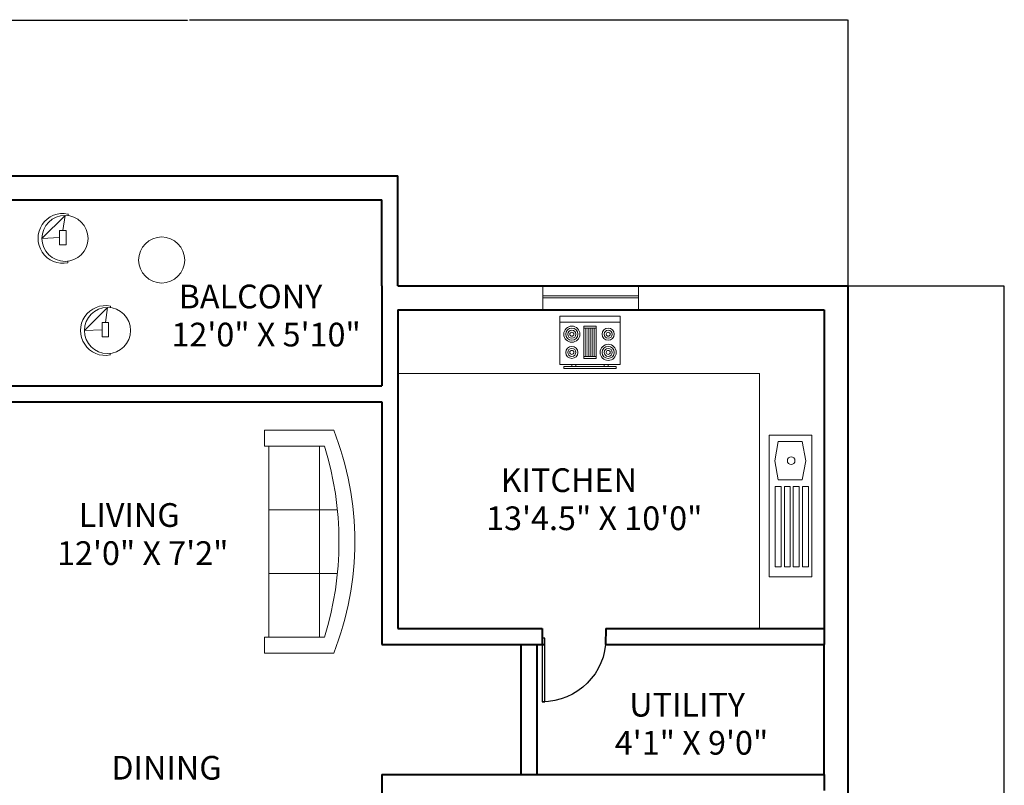
# Model space of a CAD drawing. Units: inches. Extents: x -46 to 1145, y -527 to 760.
# Tile 57 of 57: x 775 to 1145, y 472 to 760. Entities that reach past the tile are written whole.
import ezdxf

# ---------------------------------------------------------------- set-up
doc = ezdxf.new("R2010")
doc.units = ezdxf.units.IN
doc.header["$MEASUREMENT"] = 0
for name, color, linetype, lineweight in [('A-ANNO-DIMS', 2, 'Continuous', 18), ('A-AREA-IDEN', 1, 'Continuous', 18), ('A-EQPM', 2, 'Continuous', 18), ('A-FLOR-CASE', 32, 'Continuous', 18), ('A-FLOR-FIXT', 9, 'Continuous', 18), ('A-FURN', 2, 'Continuous', 13), ('DOORS', 3, 'Continuous', 25), ('WALLS', 4, 'Continuous', 40), ('WINDOWS', 240, 'Continuous', 20)]:
    doc.layers.add(name, color=color, linetype=linetype, lineweight=lineweight)
doc.styles.get("Standard").update_dxf_attribs({"font": 'arial.ttf'})
doc.dimstyles.get("Standard").update_dxf_attribs({"dimtxt": 0.18, "dimasz": 0.18, "dimexe": 0.18, "dimexo": 0.0625, "dimgap": 0.09, "dimtad": 0, "dimtih": 1, "dimtoh": 1, "dimdec": 0, "dimzin": 0, "dimdsep": 46, "dimlunit": 3, "dimtxsty": 'Standard', "dimcen": 0.09, "dimadec": 0, "dimazin": 0, "dimtfac": 1, "dimtdec": 0, "dimtofl": 0, "dimtmove": 0, "dimatfit": 3, "dimfxl": 1, "dimtolj": 1, "dimtzin": 0, "dimarcsym": 0})

# ---------------------------------------------------------------- blocks, each defined once
blk = doc.blocks.new('*U2')
for p, q in [((0, 0), (0, -6)), ((40, 0), (40, -6))]:
    blk.add_line(p, q)
blk.add_lwpolyline([(0, 0), (0, 40), (1.75, 40), (1.75, 0)], close=True)
blk.add_arc((0, 0), 40, 0, 90)
blk = doc.blocks.new('Range-Oven - 30 in top')
for p, q in [((0, -3), (30, -3)), ((12, -6), (18, -6)), ((13, -20), (13, -6)), ((14, -6), (14, -20)), ((15, -20), (15, -6)), ((16, -6), (16, -20)), ((17, -20), (17, -6)), ((6, -24), (6, -25)), ((8, -25), (8, -24)), ((18, -20), (12, -20)), ((22, -25), (22, -24)), ((24, -24), (24, -25))]:
    blk.add_line(p, q)
for points in [[(0, -24), (0, 0), (30, 0), (30, -24)], [(12, -21), (12, -5), (18, -5), (18, -21)], [(2, -26), (2, -25), (28, -25), (28, -26)]]:
    blk.add_lwpolyline(points, close=True)
for centre, radius in [((6, -9), 4), ((6, -9), 3), ((6, -9), 2), ((6, -9), 1), ((24, -9), 3), ((24, -9), 2), ((24, -9), 1), ((24, -18), 4), ((6, -18), 3), ((6, -18), 2), ((6, -18), 1), ((24, -18), 3), ((24, -18), 2), ((24, -18), 1)]:
    blk.add_circle(centre, radius)
blk = doc.blocks.new('Sofa - Roundback 7 ft.')
for p, q in [((-12.00002, -32.4421), (-12.00003, -6.5971)), ((11.99997, -32.4421), (11.99998, -6.5971)), ((-36.000027, -34), (-36.000027, -11.4696)), ((-35.999844, -13.3819), (35.9998, -13.3819)), ((35.99998, -34), (35.99998, -11.4696)), ((-36.000027, -32.4421), (35.99998, -32.4421))]:
    blk.add_line(p, q)
for points in [[(-36.000027, -34), (-42.000027, -34), (-42.000027, -8)], [(41.99998, -8), (41.99998, -34), (35.99998, -34)]]:
    blk.add_lwpolyline(points)
for centre, radius, start, end in [((0, -114.25), 114.25, 68.43141, 111.5686), ((-0.00001, -127.1968), 121.1968, 72.72033, 107.2797)]:
    blk.add_arc(centre, radius, start, end)
blk = doc.blocks.new('SINK-DRAINBOARD')
for p, q in [((3.38, 50.9), (2.09, 43.74)), ((12.47, 50.9), (13.77, 43.74)), ((3.38, 36.58), (2.09, 43.74)), ((12.47, 36.58), (13.77, 43.74))]:
    blk.add_line(p, q)
for points in [[(16.07, 0), (0, 0), (0, 53.35), (16.07, 53.35)], [(4.51, 3.73), (2.3, 3.73), (2.3, 34.08), (4.51, 34.08)], [(7.92, 3.73), (5.72, 3.73), (5.72, 34.08), (7.92, 34.08)], [(11.26, 3.73), (9.05, 3.73), (9.05, 34.08), (11.26, 34.08)], [(14.8, 3.73), (12.59, 3.73), (12.59, 34.08), (14.8, 34.08)]]:
    blk.add_lwpolyline(points, close=True)
for points in [[(3.38, 50.9), (12.47, 50.9)], [(12.47, 36.58), (3.38, 36.58)]]:
    blk.add_lwpolyline(points)
blk.add_circle((8.28, 43.74), 1.44)
blk = doc.blocks.new('BALCONY-CHAIR')
for p, q in [((11.28, 17.97), (11.28, 18.57)), ((1.49, 9.38), (10.16, 18.05)), ((9.33, 12.41), (10.16, 18.05)), ((8.08, 9.69), (1.49, 9.38)), ((11.2, 0.17), (11.2, 0.77))]:
    blk.add_line(p, q)
blk.add_lwpolyline([(10.57, 6.97), (8.08, 6.97), (8.08, 12.41), (10.57, 12.41)], close=True)
blk.add_circle((10.16, 9.38), 8.67)
blk.add_arc((9.38, 9.38), 9.38, 78.3491, 281.1485)
blk = doc.blocks.new('WINDOW-36IN')
for p, q in [((0, 4.5), (0, 9)), ((0, 9), (0, 0)), ((36, 9), (36, 0)), ((0, 5.23), (36, 5.23)), ((0, 4.5), (36, 4.5))]:
    blk.add_line(p, q)
blk = doc.blocks.new('KITCHEN-COUNTER-L')
for p, q in [((136.17, 96), (0, 96)), ((136.17, 24), (136.17, 96)), ((136.17, 0), (136.17, 24))]:
    blk.add_line(p, q)
blk = doc.blocks.new('*D686')
at = {"layer": 'A-ANNO-DIMS', "color": 0, "lineweight": -2, "transparency": 16777216}
for p, q in [((590.06, 659.58), (590.06, 759.67)), ((1086.56, 659.58), (1086.56, 759.67)), ((590.24, 759.49), (837.92, 759.49)), ((1086.38, 759.49), (838.71, 759.49))]:
    blk.add_line(p, q, dxfattribs=at)
at = {"layer": 'A-ANNO-DIMS', "color": 0, "transparency": 16777216}
for points in [[(590.24, 759.52), (590.24, 759.46), (590.06, 759.49)], [(1086.38, 759.52), (1086.38, 759.46), (1086.56, 759.49)]]:
    blk.add_solid(points, dxfattribs=at)
at = {"layer": 'Defpoints', "color": 0, "transparency": 16777216}
for p in [(1086.56, 759.49), (590.06, 659.52), (1086.56, 659.52)]:
    blk.add_point(p, dxfattribs=at)
at = {"layer": 'A-ANNO-DIMS', "color": 0, "transparency": 16777216, "insert": (838.31, 759.49), "char_height": 0.18, "attachment_point": 5}
blk.add_mtext('\\A1;496.5', dxfattribs=at)
blk = doc.blocks.new('*D688')
at = {"layer": 'A-ANNO-DIMS', "color": 0, "lineweight": -2, "transparency": 16777216}
for p, q in [((1086.63, 659.52), (1145.34, 659.52)), ((1145.16, 659.34), (1145.16, 440.7)), ((1145.16, 221.7), (1145.16, 440.34)), ((1086.63, 221.52), (1145.34, 221.52))]:
    blk.add_line(p, q, dxfattribs=at)
at = {"layer": 'A-ANNO-DIMS', "color": 0, "transparency": 16777216}
for points in [[(1145.13, 659.34), (1145.19, 659.34), (1145.16, 659.52)], [(1145.13, 221.7), (1145.19, 221.7), (1145.16, 221.52)]]:
    blk.add_solid(points, dxfattribs=at)
at = {"layer": 'Defpoints', "color": 0, "transparency": 16777216}
for p in [(1086.56, 659.52), (1145.16, 659.52), (1086.56, 221.52)]:
    blk.add_point(p, dxfattribs=at)
at = {"layer": 'A-ANNO-DIMS', "color": 0, "transparency": 16777216, "insert": (1145.16, 440.52), "char_height": 0.18, "attachment_point": 5}
blk.add_mtext('\\A1;438', dxfattribs=at)

msp = doc.modelspace()

# ---------------------------------------------------------------- linework, layer by layer
at = {"layer": 'A-FURN'}
msp.add_circle((828.2515, 669.2086), 8.6686, dxfattribs=at)
at = {"layer": 'WALLS'}
for p, q in [((767.0637, 700.8886), (917.0637, 700.8886)), ((917.0637, 659.5176), (917.0637, 700.8886)), ((767.0637, 691.8886), (911.0637, 691.8886)), ((911.0637, 659.5176), (911.0637, 691.8886)), ((911.0637, 659.5176), (911.0637, 621.8886)), ((917.0637, 659.5176), (1086.5637, 659.5176)), ((1086.5637, 221.5176), (1086.5637, 659.5176)), ((917.0637, 650.5176), (917.0637, 530.5176)), ((917.0637, 650.5176), (1077.5637, 650.5176)), ((1077.5637, 650.5176), (1077.5637, 524.5176)), ((761.0637, 621.8886), (911.0637, 621.8886)), ((761.0637, 615.8886), (911.0637, 615.8886)), ((911.0637, 615.8886), (911.0637, 524.5176)), ((917.0637, 530.5176), (971.4282, 530.5176)), ((971.4282, 530.5176), (971.4282, 524.5176)), ((995.4282, 530.5176), (995.3079, 524.5176)), ((995.4282, 530.5176), (1077.5637, 530.5176)), ((911.0637, 524.5176), (972.4782, 524.5176)), ((963.5637, 475.5176), (963.5637, 524.5176)), ((969.5637, 475.5176), (969.5637, 524.5176)), ((995.3079, 524.5176), (1077.5637, 524.5176)), ((1077.5637, 475.5176), (1077.5637, 524.5176)), ((911.0637, 475.5176), (911.0637, 367.232)), ((911.0637, 475.5176), (1077.5637, 475.5176)), ((1077.5637, 475.5176), (1077.5637, 469.5176))]:
    msp.add_line(p, q, dxfattribs=at)

# ---------------------------------------------------------------- block references
at = {"layer": 'A-EQPM', "xscale": 0.7600381531222953, "yscale": 0.7600381531222953, "zscale": 0.7600381531222953}
msp.add_blockref('Range-Oven - 30 in top', (978.0568, 648.1251), dxfattribs=at)
at = {"layer": 'A-FLOR-CASE'}
msp.add_blockref('KITCHEN-COUNTER-L', (917.064, 530.518), dxfattribs=at)
at = {"layer": 'A-FLOR-FIXT'}
msp.add_blockref('SINK-DRAINBOARD', (1056.873, 549.944), dxfattribs=at)
at = {"layer": 'A-FURN'}
for p in [(781.715, 667.966), (797.7165, 633.2915)]:
    msp.add_blockref('BALCONY-CHAIR', p, dxfattribs=at)
at = {"layer": 'A-FURN', "rotation": 270}
msp.add_blockref('Sofa - Roundback 7 ft.', (900.983, 563.2097), dxfattribs=at)
at = {"layer": 'DOORS', "xscale": -0.6, "yscale": 0.6, "zscale": 0.6, "rotation": 180}
msp.add_blockref('*U2', (971.4282, 526.9176), dxfattribs=at)
at = {"layer": 'WINDOWS'}
msp.add_blockref('WINDOW-36IN', (971.6543, 650.518), dxfattribs=at)

# ---------------------------------------------------------------- texts
at = {"layer": 'A-AREA-IDEN'}
for s, height, p in [(' BALCONY', 8.92326, (831.917, 651.021)), ('12\'0" X 5\'10"', 8.923264, (831.917, 636.6866)), ('  KITCHEN', 8.92326, (950.3531, 581.8845)), ('   LIVING', 8.92326, (788.8696, 568.7716)), ('13\'4.5" X 10\'0"', 8.923264, (950.3531, 567.5501)), ('12\'0" X 7\'2"', 8.923264, (788.8696, 554.4372)), ('   UTILITY', 8.92326, (996.0384, 497.3824)), (' 4\'1" X 9\'0"', 8.923264, (996.0384, 483.0479)), ('   DINING', 8.92326, (801.1059, 473.6409))]:
    msp.add_text(s, height=height, dxfattribs=at).set_placement(p)

# ---------------------------------------------------------------- dimensions: what is measured, and where the dimension line sits
at = {"layer": 'A-ANNO-DIMS'}
dim = msp.add_linear_dim(base=(1086.5637, 759.4886), p1=(590.0637, 659.5176), p2=(1086.5637, 659.5176), dimstyle='Standard', override={"dimdec": 1, "dimlfac": 1, "dimrnd": 0, "dimzin": 0, "dimdsep": 46, "dimlunit": 2}, dxfattribs=at)
dim.commit()
dim.dimension.update_dxf_attribs({"geometry": '*D686', "text_midpoint": (838.3137, 759.4886)})
dim = msp.add_linear_dim(base=(1145.1637, 659.5176), p1=(1086.5637, 221.5176), p2=(1086.5637, 659.5176), angle=90, dimstyle='Standard', override={"dimdec": 0, "dimlfac": 1, "dimrnd": 0, "dimzin": 0, "dimdsep": 46, "dimlunit": 2}, dxfattribs=at)
dim.commit()
dim.dimension.update_dxf_attribs({"geometry": '*D688', "text_midpoint": (1145.1637, 440.5176)})

doc.saveas('drawing.dxf')
